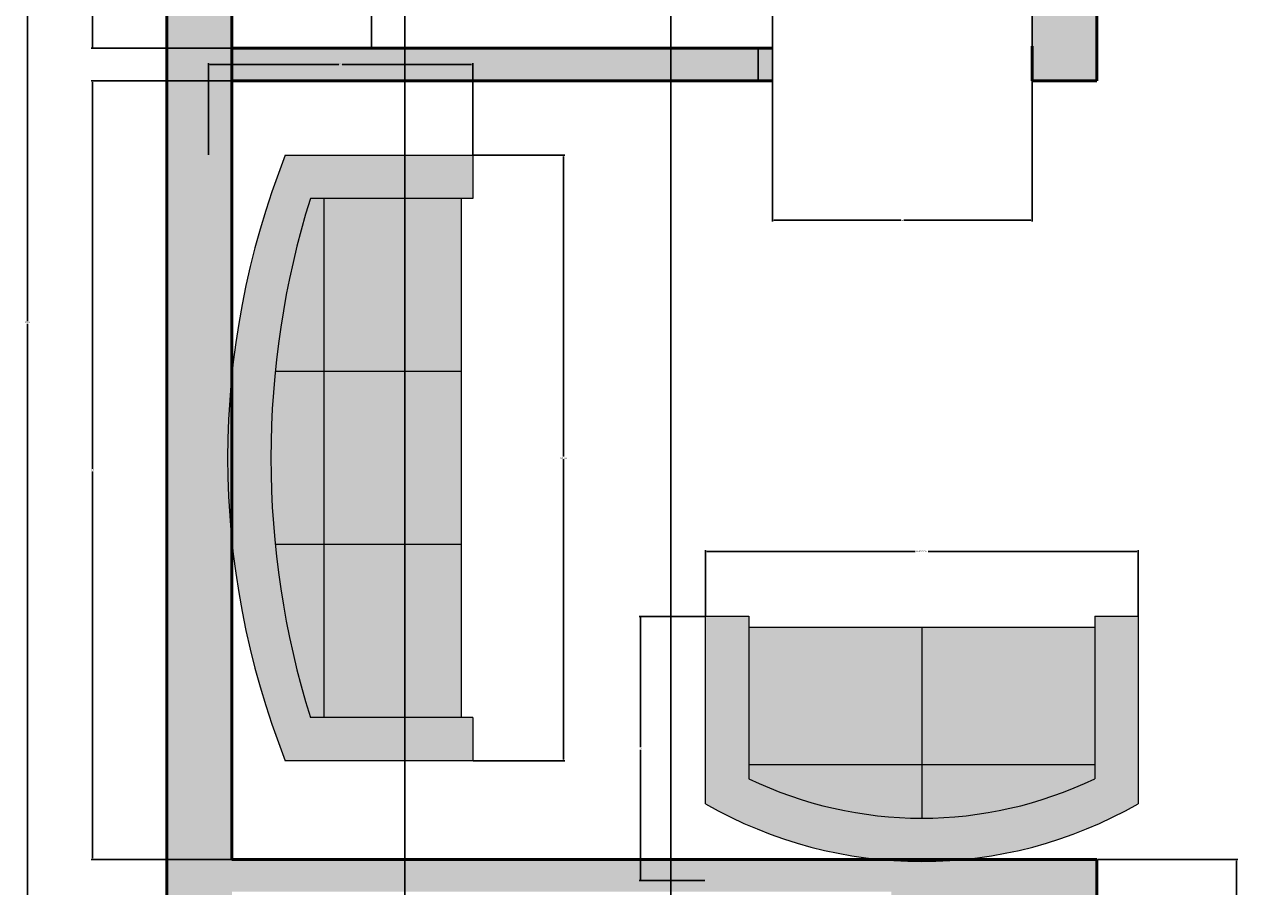
# Model space of a CAD drawing. Units: inches. Extents: x 2578 to 2919, y 51 to 451.
# Tile 2 of 5: x 2578 to 2750, y 174 to 293. Entities that reach past the tile are written whole.
import ezdxf

# ---------------------------------------------------------------- set-up
doc = ezdxf.new("R2010")
doc.units = ezdxf.units.IN
for name, color, linetype, lineweight in [('A-ANNO-DIMS', 2, 'Continuous', 18), ('A-DOOR', 4, 'Continuous', 25), ('A-FURN', 8, 'Continuous', 18), ('A-FURN-PATT', 253, 'Continuous', 13), ('A-WALL', 7, 'Continuous', 50), ('A-WALL-PATT', 250, 'Continuous', 13)]:
    doc.layers.add(name, color=color, linetype=linetype, lineweight=lineweight)
doc.layers.add('A-DOOR-PATT', color=29, linetype='Continuous', lineweight=13, true_color=0x4f342a)
doc.styles.get("Standard").update_dxf_attribs({"font": 'arial.ttf'})
doc.dimstyles.get("Standard").update_dxf_attribs({"dimtxt": 0.18, "dimasz": 0.18, "dimexe": 0.18, "dimexo": 0.0625, "dimgap": 0.09, "dimtad": 0, "dimtih": 1, "dimtoh": 1, "dimdec": 4, "dimzin": 0, "dimdsep": 46, "dimtxsty": 'Standard', "dimcen": 0.09, "dimadec": 0, "dimazin": 0, "dimtfac": 1, "dimtdec": 4, "dimtofl": 0, "dimtmove": 0, "dimatfit": 3, "dimfxl": 1, "dimtolj": 1, "dimtzin": 0, "dimarcsym": 0})

# ---------------------------------------------------------------- blocks, each defined once
blk = doc.blocks.new('*U2')
for p, q in [((0, 0), (0, -6)), ((-40, 0), (-40, -6))]:
    blk.add_line(p, q)
blk.add_lwpolyline([(0, 0), (0, 40), (-1.75, 40), (-1.75, 0)], close=True)
blk.add_arc((0, 0), 40, 90, 180)
blk = doc.blocks.new('Sofa - Roundback Loveseat 5 ft.')
for p, q in [((0, -32.44198), (0, -5.99998)), ((-24, -33.99998), (-24, -11.46958)), ((24.00004, -33.99998), (24.00004, -11.46958)), ((-23.9998, -13.38178), (23.99986, -13.38178)), ((-24, -32.44198), (24.00004, -32.44198))]:
    blk.add_line(p, q)
for points in [[(-24, -33.99998), (-30, -33.99998), (-30, -7.99998)], [(30.00004, -7.99998), (30.00004, -33.99998), (24.00004, -33.99998)]]:
    blk.add_lwpolyline(points)
for centre, radius, start, end in [((0, -60.24998), 60.24998, 60.13715, 119.8628), ((0, -61.38438), 55.38444, 64.32083, 115.6792)]:
    blk.add_arc(centre, radius, start, end)
blk = doc.blocks.new('Sofa - Roundback 7 ft.')
for p, q in [((-12.00002, -32.4421), (-12.00003, -6.5971)), ((11.99997, -32.4421), (11.99998, -6.5971)), ((-36.000027, -34), (-36.000027, -11.4696)), ((35.99998, -34), (35.99998, -11.4696)), ((-35.999844, -13.3819), (35.9998, -13.3819)), ((-36.000027, -32.4421), (35.99998, -32.4421))]:
    blk.add_line(p, q)
for points in [[(-36.000027, -34), (-42.000027, -34), (-42.000027, -8)], [(41.99998, -8), (41.99998, -34), (35.99998, -34)]]:
    blk.add_lwpolyline(points)
for centre, radius, start, end in [((0, -114.25), 114.25, 68.43141, 111.5686), ((-0.00001, -127.1968), 121.1968, 72.72033, 107.2797)]:
    blk.add_arc(centre, radius, start, end)
blk = doc.blocks.new('*D25')
at = {"layer": 'A-ANNO-DIMS', "color": 0, "lineweight": -2, "transparency": 16777216}
for p, q in [((2672.25, 211.42), (2672.25, 220.53)), ((2672.43, 220.35), (2701.33, 220.35)), ((2732.07, 220.35), (2703.16, 220.35)), ((2732.25, 211.42), (2732.25, 220.53))]:
    blk.add_line(p, q, dxfattribs=at)
at = {"layer": 'A-ANNO-DIMS', "color": 0, "transparency": 16777216}
for points in [[(2672.43, 220.38), (2672.43, 220.32), (2672.25, 220.35)], [(2732.07, 220.38), (2732.07, 220.32), (2732.25, 220.35)]]:
    blk.add_solid(points, dxfattribs=at)
at = {"layer": 'Defpoints', "color": 0, "transparency": 16777216}
for p in [(2672.25, 220.35), (2672.25, 211.35), (2732.25, 211.35)]:
    blk.add_point(p, dxfattribs=at)
at = {"layer": 'A-ANNO-DIMS', "color": 0, "transparency": 16777216, "insert": (2702.25, 220.35), "char_height": 0.18, "attachment_point": 5}
blk.add_mtext('\\A1;LOVESEAT 60', dxfattribs=at)
blk = doc.blocks.new('*D26')
at = {"layer": 'A-ANNO-DIMS', "color": 0, "lineweight": -2, "transparency": 16777216}
for p, q in [((2672.18, 211.35), (2663.07, 211.35)), ((2663.25, 211.17), (2663.25, 193.2)), ((2663.25, 174.87), (2663.25, 192.84)), ((2672.18, 174.69), (2663.07, 174.69))]:
    blk.add_line(p, q, dxfattribs=at)
at = {"layer": 'A-ANNO-DIMS', "color": 0, "transparency": 16777216}
for points in [[(2663.22, 211.17), (2663.28, 211.17), (2663.25, 211.35)], [(2663.22, 174.87), (2663.28, 174.87), (2663.25, 174.69)]]:
    blk.add_solid(points, dxfattribs=at)
at = {"layer": 'Defpoints', "color": 0, "transparency": 16777216}
for p in [(2672.25, 211.35), (2663.25, 174.69), (2672.25, 174.69)]:
    blk.add_point(p, dxfattribs=at)
at = {"layer": 'A-ANNO-DIMS', "color": 0, "transparency": 16777216, "insert": (2663.25, 193.02), "char_height": 0.18, "attachment_point": 5}
blk.add_mtext('\\A1;37', dxfattribs=at)
blk = doc.blocks.new('*D29')
at = {"layer": 'A-ANNO-DIMS', "color": 0, "lineweight": -2, "transparency": 16777216}
for p, q in [((2640.03, 275.32), (2652.75, 275.32)), ((2652.57, 275.14), (2652.57, 233.5)), ((2652.57, 191.5), (2652.57, 233.13)), ((2640.03, 191.32), (2652.75, 191.32))]:
    blk.add_line(p, q, dxfattribs=at)
at = {"layer": 'A-ANNO-DIMS', "color": 0, "transparency": 16777216}
for points in [[(2652.54, 275.14), (2652.6, 275.14), (2652.57, 275.32)], [(2652.54, 191.5), (2652.6, 191.5), (2652.57, 191.32)]]:
    blk.add_solid(points, dxfattribs=at)
at = {"layer": 'Defpoints', "color": 0, "transparency": 16777216}
for p in [(2639.97, 275.32), (2652.57, 275.32), (2639.97, 191.32)]:
    blk.add_point(p, dxfattribs=at)
at = {"layer": 'A-ANNO-DIMS', "color": 0, "transparency": 16777216, "insert": (2652.57, 233.32), "char_height": 0.18, "attachment_point": 5}
blk.add_mtext('\\A1;SOFA 84', dxfattribs=at)
blk = doc.blocks.new('*D30')
at = {"layer": 'A-ANNO-DIMS', "color": 0, "lineweight": -2, "transparency": 16777216}
for p, q in [((2603.3, 275.38), (2603.3, 288.1)), ((2603.48, 287.92), (2621.41, 287.92)), ((2639.79, 287.92), (2621.85, 287.92)), ((2639.97, 275.38), (2639.97, 288.1))]:
    blk.add_line(p, q, dxfattribs=at)
at = {"layer": 'A-ANNO-DIMS', "color": 0, "transparency": 16777216}
for points in [[(2603.48, 287.95), (2603.48, 287.89), (2603.3, 287.92)], [(2639.79, 287.95), (2639.79, 287.89), (2639.97, 287.92)]]:
    blk.add_solid(points, dxfattribs=at)
at = {"layer": 'Defpoints', "color": 0, "transparency": 16777216}
for p in [(2603.3, 287.92), (2603.3, 275.32), (2639.97, 275.32)]:
    blk.add_point(p, dxfattribs=at)
at = {"layer": 'A-ANNO-DIMS', "color": 0, "transparency": 16777216, "insert": (2621.63, 287.92), "char_height": 0.18, "attachment_point": 5}
blk.add_mtext('\\A1;37', dxfattribs=at)
blk = doc.blocks.new('*D36')
at = {"layer": 'A-ANNO-DIMS', "color": 0, "lineweight": -2, "transparency": 16777216}
for p, q in [((2597.48, 431.14), (2578.02, 431.14)), ((2578.2, 430.96), (2578.2, 252.3)), ((2578.2, 73.28), (2578.2, 251.94)), ((2597.48, 73.1), (2578.02, 73.1))]:
    blk.add_line(p, q, dxfattribs=at)
at = {"layer": 'A-ANNO-DIMS', "color": 0, "transparency": 16777216}
for points in [[(2578.17, 430.96), (2578.23, 430.96), (2578.2, 431.14)], [(2578.17, 73.28), (2578.23, 73.28), (2578.2, 73.1)]]:
    blk.add_solid(points, dxfattribs=at)
at = {"layer": 'Defpoints', "color": 0, "transparency": 16777216}
for p in [(2578.2, 431.14), (2597.55, 431.14), (2597.55, 73.1)]:
    blk.add_point(p, dxfattribs=at)
at = {"layer": 'A-ANNO-DIMS', "color": 0, "transparency": 16777216, "insert": (2578.2, 252.12), "char_height": 0.18, "attachment_point": 5}
blk.add_mtext('\\A1;358.04', dxfattribs=at)
blk = doc.blocks.new('*D40')
at = {"layer": 'A-ANNO-DIMS', "color": 0, "lineweight": -2, "transparency": 16777216}
for p, q in [((2606.48, 422.14), (2587.02, 422.14)), ((2587.2, 421.96), (2587.2, 356.32)), ((2587.2, 290.32), (2587.2, 355.96)), ((2606.48, 290.14), (2587.02, 290.14))]:
    blk.add_line(p, q, dxfattribs=at)
at = {"layer": 'A-ANNO-DIMS', "color": 0, "transparency": 16777216}
for points in [[(2587.17, 421.96), (2587.23, 421.96), (2587.2, 422.14)], [(2587.17, 290.32), (2587.23, 290.32), (2587.2, 290.14)]]:
    blk.add_solid(points, dxfattribs=at)
at = {"layer": 'Defpoints', "color": 0, "transparency": 16777216}
for p in [(2587.2, 422.14), (2606.55, 422.14), (2606.55, 290.14)]:
    blk.add_point(p, dxfattribs=at)
at = {"layer": 'A-ANNO-DIMS', "color": 0, "transparency": 16777216, "insert": (2587.2, 356.14), "char_height": 0.18, "attachment_point": 5}
blk.add_mtext('\\A1;132', dxfattribs=at)
blk = doc.blocks.new('*D42')
at = {"layer": 'A-ANNO-DIMS', "color": 0, "lineweight": -2, "transparency": 16777216}
for p, q in [((2606.48, 285.64), (2587.02, 285.64)), ((2587.2, 285.46), (2587.2, 231.82)), ((2587.2, 177.82), (2587.2, 231.46)), ((2606.48, 177.64), (2587.02, 177.64))]:
    blk.add_line(p, q, dxfattribs=at)
at = {"layer": 'A-ANNO-DIMS', "color": 0, "transparency": 16777216}
for points in [[(2587.17, 285.46), (2587.23, 285.46), (2587.2, 285.64)], [(2587.17, 177.82), (2587.23, 177.82), (2587.2, 177.64)]]:
    blk.add_solid(points, dxfattribs=at)
at = {"layer": 'Defpoints', "color": 0, "transparency": 16777216}
for p in [(2587.2, 285.64), (2606.55, 285.64), (2606.55, 177.64)]:
    blk.add_point(p, dxfattribs=at)
at = {"layer": 'A-ANNO-DIMS', "color": 0, "transparency": 16777216, "insert": (2587.2, 231.64), "char_height": 0.18, "attachment_point": 5}
blk.add_mtext('\\A1;108', dxfattribs=at)
blk = doc.blocks.new('*D52')
at = {"layer": 'A-ANNO-DIMS', "color": 0, "lineweight": -2, "transparency": 16777216}
for p, q in [((2681.55, 285.58), (2681.55, 266.11)), ((2717.55, 285.58), (2717.55, 266.11)), ((2681.73, 266.29), (2699.33, 266.29)), ((2717.37, 266.29), (2699.77, 266.29))]:
    blk.add_line(p, q, dxfattribs=at)
at = {"layer": 'A-ANNO-DIMS', "color": 0, "transparency": 16777216}
for points in [[(2681.73, 266.32), (2681.73, 266.26), (2681.55, 266.29)], [(2717.37, 266.32), (2717.37, 266.26), (2717.55, 266.29)]]:
    blk.add_solid(points, dxfattribs=at)
at = {"layer": 'Defpoints', "color": 0, "transparency": 16777216}
for p in [(2681.55, 285.64), (2717.55, 285.64), (2681.55, 266.29)]:
    blk.add_point(p, dxfattribs=at)
at = {"layer": 'A-ANNO-DIMS', "color": 0, "transparency": 16777216, "insert": (2699.55, 266.29), "char_height": 0.18, "attachment_point": 5}
blk.add_mtext('\\A1;36', dxfattribs=at)
blk = doc.blocks.new('*D53')
at = {"layer": 'A-ANNO-DIMS', "color": 0, "lineweight": -2, "transparency": 16777216}
for p, q in [((2606.55, 285.7), (2606.55, 305.17)), ((2606.73, 304.99), (2643.83, 304.99)), ((2681.37, 304.99), (2644.27, 304.99)), ((2681.55, 285.7), (2681.55, 305.17))]:
    blk.add_line(p, q, dxfattribs=at)
at = {"layer": 'A-ANNO-DIMS', "color": 0, "transparency": 16777216}
for points in [[(2606.73, 305.02), (2606.73, 304.96), (2606.55, 304.99)], [(2681.37, 305.02), (2681.37, 304.96), (2681.55, 304.99)]]:
    blk.add_solid(points, dxfattribs=at)
at = {"layer": 'Defpoints', "color": 0, "transparency": 16777216}
for p in [(2681.55, 304.99), (2606.55, 285.64), (2681.55, 285.64)]:
    blk.add_point(p, dxfattribs=at)
at = {"layer": 'A-ANNO-DIMS', "color": 0, "transparency": 16777216, "insert": (2644.05, 304.99), "char_height": 0.18, "attachment_point": 5}
blk.add_mtext('\\A1;75', dxfattribs=at)
blk = doc.blocks.new('*D65')
at = {"layer": 'A-ANNO-DIMS', "color": 0, "lineweight": -2, "transparency": 16777216}
for p, q in [((2726.61, 177.64), (2746.08, 177.64)), ((2745.9, 177.46), (2745.9, 167.8)), ((2745.9, 157.78), (2745.9, 167.44)), ((2726.61, 157.6), (2746.08, 157.6))]:
    blk.add_line(p, q, dxfattribs=at)
at = {"layer": 'A-ANNO-DIMS', "color": 0, "transparency": 16777216}
for points in [[(2745.87, 177.46), (2745.93, 177.46), (2745.9, 177.64)], [(2745.87, 157.78), (2745.93, 157.78), (2745.9, 157.6)]]:
    blk.add_solid(points, dxfattribs=at)
at = {"layer": 'Defpoints', "color": 0, "transparency": 16777216}
for p in [(2726.55, 177.64), (2726.55, 157.6), (2745.9, 157.6)]:
    blk.add_point(p, dxfattribs=at)
at = {"layer": 'A-ANNO-DIMS', "color": 0, "transparency": 16777216, "insert": (2745.9, 167.62), "char_height": 0.18, "attachment_point": 5}
blk.add_mtext('\\A1;20.04', dxfattribs=at)
blk = doc.blocks.new('*D70')
at = {"layer": 'A-ANNO-DIMS', "color": 0, "lineweight": -2, "transparency": 16777216}
for p, q in [((2630.55, 156.2), (2630.55, 450.67)), ((2630.73, 450.49), (2648.67, 450.49)), ((2667.27, 450.49), (2649.32, 450.49)), ((2667.45, 155.71), (2667.45, 450.67))]:
    blk.add_line(p, q, dxfattribs=at)
at = {"layer": 'A-ANNO-DIMS', "color": 0, "transparency": 16777216}
for points in [[(2630.73, 450.52), (2630.73, 450.46), (2630.55, 450.49)], [(2667.27, 450.52), (2667.27, 450.46), (2667.45, 450.49)]]:
    blk.add_solid(points, dxfattribs=at)
at = {"layer": 'Defpoints', "color": 0, "transparency": 16777216}
for p in [(2667.45, 450.49), (2630.55, 156.14), (2667.45, 155.64)]:
    blk.add_point(p, dxfattribs=at)
at = {"layer": 'A-ANNO-DIMS', "color": 0, "transparency": 16777216, "insert": (2649, 450.49), "char_height": 0.18, "attachment_point": 5}
blk.add_mtext('\\A1;36.9', dxfattribs=at)
blk = doc.blocks.new('*D72')
at = {"layer": 'A-ANNO-DIMS', "color": 0, "lineweight": -2, "transparency": 16777216}
for p, q in [((2606.65, 364.52), (2626.11, 364.51)), ((2625.93, 364.33), (2625.91, 327.5)), ((2625.9, 290.31), (2625.91, 327.14)), ((2606.61, 290.14), (2626.08, 290.13))]:
    blk.add_line(p, q, dxfattribs=at)
at = {"layer": 'A-ANNO-DIMS', "color": 0, "transparency": 16777216}
for points in [[(2625.9, 364.33), (2625.96, 364.33), (2625.93, 364.51)], [(2625.87, 290.31), (2625.93, 290.31), (2625.9, 290.13)]]:
    blk.add_solid(points, dxfattribs=at)
at = {"layer": 'Defpoints', "color": 0, "transparency": 16777216}
for p in [(2606.58, 364.52), (2606.55, 290.14), (2625.9, 290.13)]:
    blk.add_point(p, dxfattribs=at)
at = {"layer": 'A-ANNO-DIMS', "color": 0, "transparency": 16777216, "insert": (2625.91, 327.32), "char_height": 0.18, "attachment_point": 5}
blk.add_mtext('\\A1;74.38', dxfattribs=at)

msp = doc.modelspace()

# ---------------------------------------------------------------- hatches: boundary and pattern name
at = {"layer": 'A-DOOR-PATT'}
h = msp.add_hatch(color=256, dxfattribs=at)
h.dxf.hatch_style = 1
h.paths.add_polyline_path([(2717.5545, 331.5492, 0.01094143), (2715.9791, 331.5147), (2715.9791, 295.5417), (2717.5545, 295.5417)])
h.paths.add_polyline_path([(2772.7563, 343.5147, 0.01094143), (2771.181, 343.5492), (2771.181, 307.5417), (2772.7563, 307.5417)])
h.paths.add_polyline_path([(2809.181, 302.1406), (2807.181, 302.1406), (2807.181, 297.6406), (2809.181, 297.6406)])
h.paths.add_polyline_path([(2681.547, 290.1406), (2679.547, 290.1406), (2679.547, 285.6406), (2681.547, 285.6406)])
h.paths.add_polyline_path([(2870.5896, 193.5988), (2834.5821, 193.5988), (2834.5821, 192.0235), (2870.5551, 192.0235, 0.01094143)])
h.paths.add_polyline_path([(2829.181, 157.5988), (2824.681, 157.5988), (2824.681, 155.5988), (2829.181, 155.5988)])
h.paths.add_polyline_path([(2702.547, 145.6406), (2698.047, 145.6406), (2698.047, 143.6481), (2702.547, 143.6481)])
h.paths.add_polyline_path([(2697.1459, 109.2159), (2661.1384, 109.2159), (2661.1384, 107.6406), (2697.1459, 107.6406)])
h.paths.add_polyline_path([(2702.547, 107.6406), (2698.047, 107.6406), (2698.047, 105.6406), (2702.547, 105.6406)])
h.paths.add_polyline_path([(2771.181, 302.1406), (2769.181, 302.1406), (2769.181, 297.6406), (2771.181, 297.6406)])
at = {"layer": 'A-FURN-PATT'}
h = msp.add_hatch(color=256, dxfattribs=at)
h.dxf.hatch_style = 1
h.paths.add_polyline_path([(2726.2468, 209.7963), (2702.2468, 209.7963), (2702.2468, 190.7361), (2726.2468, 190.7361)], flags=17)
h.paths.add_polyline_path([(2702.2468, 209.7963), (2678.2467, 209.7963), (2678.2467, 190.7361), (2702.2468, 190.7361)], flags=17)
h.paths.add_polyline_path([(2702.2468, 190.7361), (2678.2467, 190.7361), (2678.2467, 188.8244, 0.11251889), (2702.2468, 183.3542)], flags=17)
h.paths.add_polyline_path([(2726.2468, 188.8244), (2726.2468, 190.7361), (2702.2468, 190.7361), (2702.2468, 183.3542, 0.11251869)], flags=17)
h.paths.add_polyline_path([(2732.2468, 185.3543), (2732.2468, 211.3543), (2726.2468, 211.3543), (2726.2468, 188.8244, -0.22792319), (2678.2467, 188.8244), (2678.2467, 211.3543), (2672.2467, 211.3543), (2672.2467, 185.3543, 0.10631811), (2696.3802, 177.6406), (2708.1133, 177.6406, 0.10631791)])
h.paths.add_polyline_path([(2638.4076, 269.3173), (2619.3474, 269.3173), (2619.3474, 245.3173), (2638.4076, 245.3172)], flags=17)
h.paths.add_polyline_path([(2639.9655, 275.3173), (2613.9655, 275.3173, 0.06898518), (2606.547, 244.8299), (2606.547, 221.8046, 0.06898529), (2613.9655, 191.3172), (2639.9655, 191.3172), (2639.9655, 197.3172), (2617.4356, 197.3172, -0.15194781), (2617.4356, 269.3173), (2639.9655, 269.3173)])
h.paths.add_polyline_path([(2619.3474, 269.3173), (2617.4356, 269.3173, 0.05064665), (2612.561, 245.3173), (2619.3474, 245.3173)], flags=17)
h.paths.add_polyline_path([(2619.3474, 245.3173), (2612.561, 245.3173, 0.04962821), (2612.561, 221.3172), (2619.3474, 221.3172)], flags=17)
h.paths.add_polyline_path([(2638.4076, 245.3172), (2619.3474, 245.3173), (2619.3474, 221.3172), (2638.4076, 221.3173)], flags=17)
h.paths.add_polyline_path([(2638.4076, 221.3173), (2619.3474, 221.3172), (2619.3474, 197.3172), (2638.4076, 197.3172)], flags=17)
h.paths.add_polyline_path([(2619.3474, 221.3172), (2612.561, 221.3172, 0.05064665), (2617.4356, 197.3172), (2619.3474, 197.3172)], flags=17)
at = {"layer": 'A-WALL-PATT'}
h = msp.add_hatch(color=256, dxfattribs=at)
h.dxf.hatch_style = 1
h.paths.add_polyline_path([(2606.547, 422.1406), (2889.181, 422.1406), (2889.181, 210.611), (2824.681, 210.611), (2824.681, 193.5988), (2829.181, 193.5988), (2829.181, 206.111), (2889.181, 206.111), (2889.181, 99.5988), (2829.181, 99.5988), (2829.181, 155.5988), (2824.681, 155.5988), (2824.681, 95.0988), (2889.181, 95.0988), (2889.181, 82.1022), (2762.547, 82.1022), (2762.547, 73.1022), (2898.181, 73.1022), (2898.181, 233.1022), (2898.181, 431.1406), (2597.547, 431.1406), (2597.547, 73.1022), (2726.547, 73.1022), (2726.547, 82.1022), (2606.547, 82.1022), (2606.547, 173.1406), (2698.047, 173.1406), (2698.047, 145.6406), (2702.547, 145.6406), (2702.547, 157.5988), (2726.547, 157.5988), (2726.547, 177.6406), (2606.547, 177.6406)])
h.paths.add_polyline_path([(2889.181, 302.1406), (2809.181, 302.1406), (2809.181, 297.6406), (2889.181, 297.6406)], flags=17)
h.paths.add_polyline_path([(2679.547, 290.1406), (2606.547, 290.1406), (2606.547, 285.6406), (2679.547, 285.6406)], flags=17)
h.paths.add_polyline_path([(2824.681, 157.5988), (2800.681, 157.5988), (2800.681, 155.5988), (2824.681, 155.5988)], flags=17)
h.paths.add_polyline_path([(2698.047, 105.6406), (2606.547, 105.6406), (2606.547, 101.1406), (2698.047, 101.1406)], flags=17)
h.paths.add_polyline_path([(2702.547, 105.6406), (2698.047, 105.6406), (2698.047, 101.1406), (2702.547, 101.1406)], flags=17)
h.paths.add_polyline_path([(2726.547, 422.1406), (2722.047, 422.1406), (2722.047, 295.5417), (2717.5545, 295.5417), (2717.5545, 290.1406), (2717.5504, 285.6406), (2722.047, 285.6406), (2726.547, 285.6406)], flags=17)
h.paths.add_polyline_path([(2769.181, 422.1406), (2764.681, 422.1406), (2764.681, 297.6406), (2769.181, 297.6406)], flags=17)

# ---------------------------------------------------------------- linework, layer by layer
at = {"layer": 'A-DOOR'}
for p, q in [((2679.547, 285.6406), (2679.547, 290.1406)), ((2681.547, 285.6406), (2681.547, 290.1406))]:
    msp.add_line(p, q, dxfattribs=at)
at = {"layer": 'A-WALL'}
for p, q in [((2606.547, 177.6406), (2606.547, 422.1406)), ((2726.547, 285.6406), (2726.547, 422.1406)), ((2717.5504, 285.6406), (2717.5545, 290.4444)), ((2606.547, 290.1406), (2681.547, 290.1406)), ((2606.547, 285.6406), (2681.547, 285.6406)), ((2722.047, 285.6406), (2717.5504, 285.6406)), ((2722.047, 285.6406), (2726.547, 285.6406)), ((2606.547, 177.6406), (2726.547, 177.6406)), ((2726.547, 157.5988), (2726.547, 177.6406))]:
    msp.add_line(p, q, dxfattribs=at)
msp.add_lwpolyline([(2726.547, 73.1022), (2597.547, 73.1022), (2597.547, 431.1406), (2898.181, 431.1406), (2898.181, 233.1022), (2898.181, 73.1022), (2762.547, 73.1022)], dxfattribs=at)

# ---------------------------------------------------------------- block references
at = {"layer": 'A-DOOR', "xscale": 0.9001866182309679, "yscale": 0.9001866182309679, "zscale": 0.9001866182309679}
msp.add_blockref('*U2', (2717.5545, 295.5417), dxfattribs=at)
at = {"layer": 'A-FURN'}
for name, p, rotation in [('Sofa - Roundback 7 ft.', (2605.9655, 233.3173), 90), ('Sofa - Roundback Loveseat 5 ft.', (2702.2468, 177.3543), 180)]:
    msp.add_blockref(name, p, dxfattribs=dict(at, rotation=rotation))

# ---------------------------------------------------------------- dimensions: what is measured, and where the dimension line sits
at = {"layer": 'A-ANNO-DIMS'}
dim = msp.add_linear_dim(base=(2667.4454, 450.4906), p1=(2630.547, 156.1406), p2=(2667.4454, 155.6436), dimstyle='Standard', override={"dimdec": 1, "dimlfac": 1, "dimrnd": 0, "dimzin": 0, "dimdsep": 46, "dimlunit": 2}, dxfattribs=at)
dim.commit()
dim.dimension.update_dxf_attribs({"geometry": '*D70', "text_midpoint": (2648.9962, 450.4906)})
for base, p1, p2, angle, override, picture, middle in [((2578.197, 431.1406), (2597.547, 73.1022), (2597.547, 431.1406), 90, {"dimdec": 2, "dimlfac": 1, "dimrnd": 0, "dimzin": 0, "dimdsep": 46, "dimlunit": 2}, '*D36', (2578.197, 252.1214)), ((2587.197, 422.1406), (2606.547, 290.1406), (2606.547, 422.1406), 90, {"dimdec": 0, "dimlfac": 1, "dimrnd": 0, "dimzin": 0, "dimdsep": 46, "dimlunit": 2}, '*D40', (2587.197, 356.1406)), ((2625.897, 290.1314), (2606.5825, 364.5234), (2606.547, 290.1406), 269.972645, {"dimdec": 2, "dimlfac": 1, "dimrnd": 0, "dimzin": 0, "dimdsep": 46, "dimlunit": 2}, '*D72', (2625.9148, 327.3227)), ((2681.547, 304.9906), (2606.547, 285.6406), (2681.547, 285.6406), 0, {"dimdec": 0, "dimlfac": 1, "dimrnd": 0, "dimzin": 0, "dimdsep": 46, "dimlunit": 2}, '*D53', (2644.047, 304.9906)), ((2603.2988, 287.9173), (2639.9655, 275.3173), (2603.2988, 275.3173), 180, {"dimdec": 0, "dimlfac": 1, "dimrnd": 0, "dimzin": 0, "dimdsep": 46, "dimlunit": 2}, '*D30', (2621.6321, 287.9173)), ((2587.197, 285.6406), (2606.547, 177.6406), (2606.547, 285.6406), 90, {"dimdec": 0, "dimlfac": 1, "dimrnd": 0, "dimzin": 0, "dimdsep": 46, "dimlunit": 2}, '*D42', (2587.197, 231.6406)), ((2681.547, 266.2906), (2717.5504, 285.6406), (2681.547, 285.6406), 180, {"dimdec": 0, "dimlfac": 1, "dimrnd": 0, "dimzin": 0, "dimdsep": 46, "dimlunit": 2}, '*D52', (2699.5487, 266.2906)), ((2663.2467, 174.6876), (2672.2467, 211.3543), (2672.2467, 174.6876), 270, {"dimdec": 0, "dimlfac": 1, "dimrnd": 0, "dimzin": 0, "dimdsep": 46, "dimlunit": 2}, '*D26', (2663.2467, 193.021)), ((2745.897, 157.5988), (2726.547, 177.6406), (2726.547, 157.5988), 270, {"dimdec": 2, "dimlfac": 1, "dimrnd": 0, "dimzin": 0, "dimdsep": 46, "dimlunit": 2}, '*D65', (2745.897, 167.6197))]:
    dim = msp.add_linear_dim(base=base, p1=p1, p2=p2, angle=angle, dimstyle='Standard', override=override, dxfattribs=at)
    dim.commit()
    dim.dimension.update_dxf_attribs({"geometry": picture, "text_midpoint": middle})
for base, p1, p2, angle, text, picture, middle in [((2652.5655, 275.3173), (2639.9655, 191.3172), (2639.9655, 275.3173), 90, 'SOFA <>', '*D29', (2652.5655, 233.3173)), ((2672.2467, 220.3543), (2732.2468, 211.3543), (2672.2467, 211.3543), 180, 'LOVESEAT <>', '*D25', (2702.2467, 220.3543))]:
    dim = msp.add_linear_dim(base=base, p1=p1, p2=p2, angle=angle, text=text, dimstyle='Standard', override={"dimdec": 0, "dimlfac": 1, "dimrnd": 0, "dimzin": 0, "dimdsep": 46, "dimlunit": 2}, dxfattribs=at)
    dim.commit()
    dim.dimension.update_dxf_attribs({"geometry": picture, "text_midpoint": middle})

doc.saveas('drawing.dxf')
